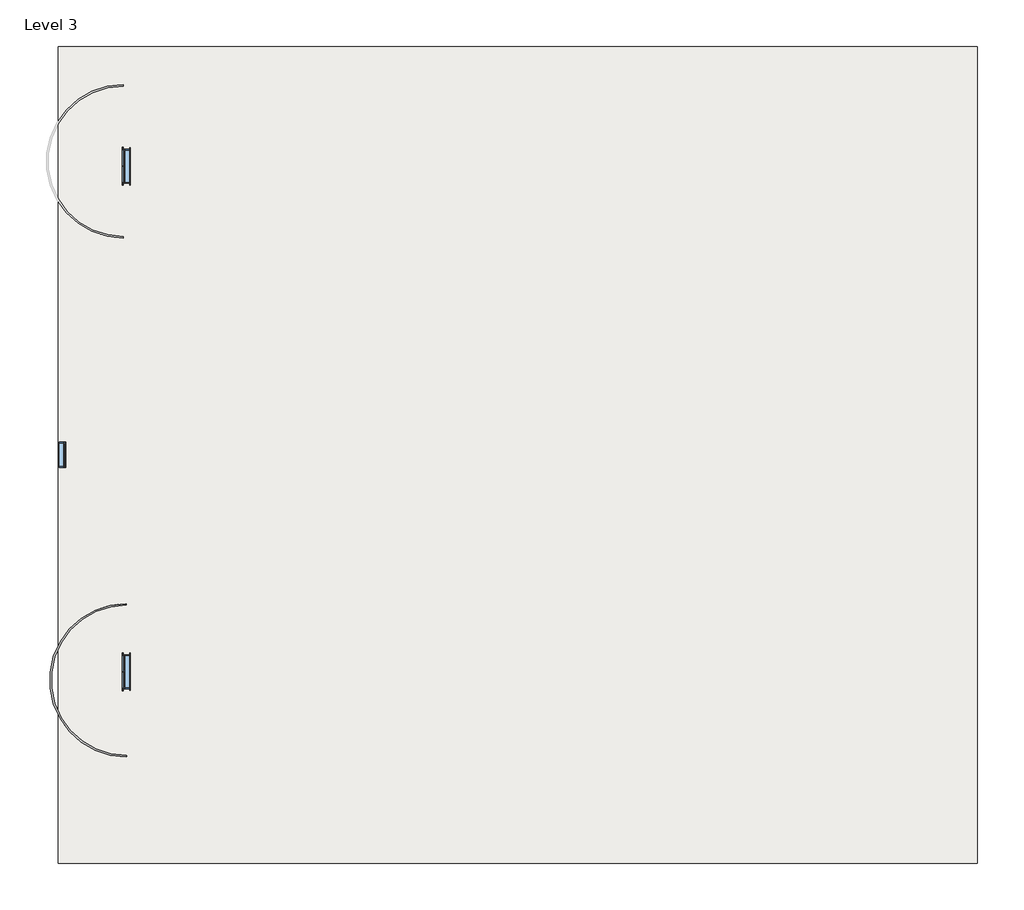
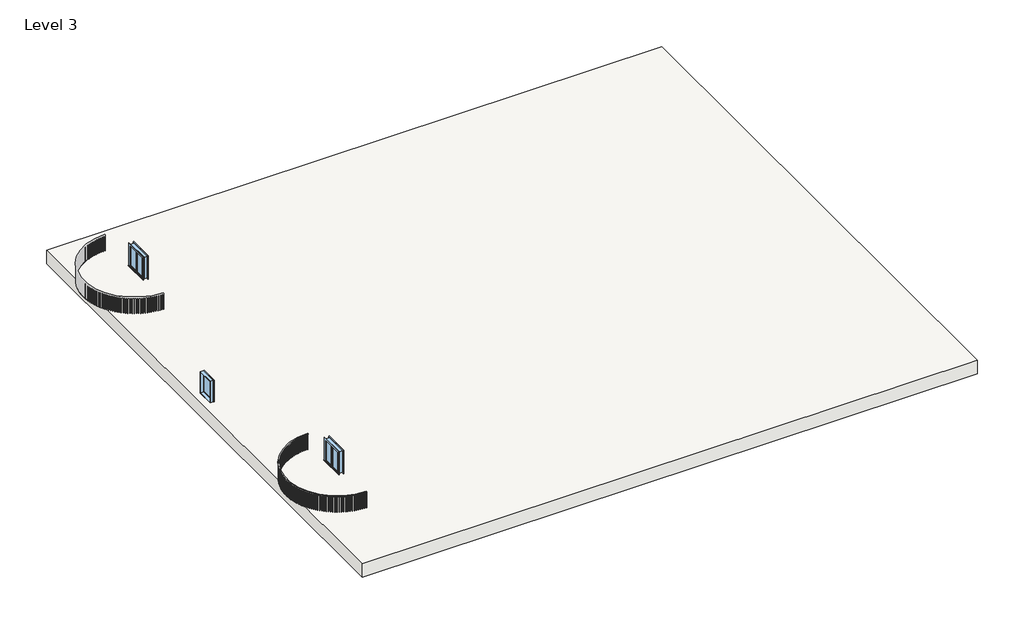
# One storey, part 1 of 2: 3 windows, 1 railing, 1 slab.
"""IFC4 building model written with IfcOpenShell, lengths in millimetres."""

from ifc_helpers import new_model, si_unit, point, frame, frame_2d, origin, place, context, project, spatial, polyline, circle_curve, trimmed, segment, composite_curve, outline, extrude, transform, mapped, element, save
from components import window_534dcd48, window_c1f32544

model = new_model("IFC4")

# Units and contexts
model_context = context("Model", 3, world=origin())
ifc_project = project(units=[si_unit("LENGTHUNIT", "METRE", prefix="MILLI")], contexts=[model_context])

# Site, building, storey
site = spatial("IfcSite", under=ifc_project)
building = spatial("IfcBuilding", under=site)
storey = spatial("IfcBuildingStorey", under=building, Name="Level 3", Elevation=6096.0)

# Railing
placement = place(None, origin())
element("IfcRailing", 1, ObjectType="Handrail - Rectangular", at=placement, inside=storey, context=model_context, shape_type="SweptSolid", body=[
    extrude(outline(composite_curve([segment(trimmed(circle_curve(frame_2d((-15613.8723021, -8267.0443987)), 2743.2), [point((-15613.8723021, -11010.2443987))], [point((-15613.8723021, -5523.8443987))], False, "CARTESIAN"), True, "CONTINUOUS"), segment(polyline([(-15613.8723021, -5523.8443987), (-15613.8723021, -5574.6443987)]), True, "CONTINUOUS"), segment(trimmed(circle_curve(frame_2d((-15613.8723021, -8267.0443987)), 2692.4), [point((-15613.8723021, -5574.6443987))], [point((-15613.8723021, -10959.4443987))], True, "CARTESIAN"), True, "CONTINUOUS"), segment(polyline([(-15613.8723021, -10959.4443987), (-15613.8723021, -11010.2443987)]), True, "CONTINUOUS")], self_intersect=False)), frame((0.0, 0.0, 6959.6), z_axis=(0.0, 0.0, 1.0), x_axis=(1.0, 0.0, 0.0)), (0.0, 0.0, 1.0), 50.8),
    extrude(outline(polyline([(-15627.231195, -10994.3533143), (-15627.2044157, -10975.3033331), (-15608.1544345, -10975.3301124), (-15608.1812138, -10994.3800936), (-15627.231195, -10994.3533143)])), frame((0.0, 0.0, 6096.0), z_axis=(0.0, 0.0, 1.0), x_axis=(1.0, 0.0, 0.0)), (0.0, 0.0, 1.0), 863.6),
    extrude(outline(polyline([(-15729.1535895, -10991.9485449), (-15728.414846, -10972.9128742), (-15709.3791753, -10973.6516178), (-15710.1179188, -10992.6872885), (-15729.1535895, -10991.9485449)])), frame((0.0, 0.0, 6096.0), z_axis=(0.0, 0.0, 1.0), x_axis=(1.0, 0.0, 0.0)), (0.0, 0.0, 1.0), 863.6),
    extrude(outline(polyline([(-15830.914897, -10985.7361601), (-15829.4652214, -10966.7413992), (-15810.4704606, -10968.1910747), (-15811.9201361, -10987.1858356), (-15830.914897, -10985.7361601)])), frame((0.0, 0.0, 6096.0), z_axis=(0.0, 0.0, 1.0), x_axis=(1.0, 0.0, 0.0)), (0.0, 0.0, 1.0), 863.6),
    extrude(outline(polyline([(-15932.3729223, -10975.7248406), (-15930.2143405, -10956.7975316), (-15911.2870315, -10958.9561134), (-15913.4456133, -10977.8834224), (-15932.3729223, -10975.7248406)])), frame((0.0, 0.0, 6096.0), z_axis=(0.0, 0.0, 1.0), x_axis=(1.0, 0.0, 0.0)), (0.0, 0.0, 1.0), 863.6),
    extrude(outline(polyline([(-16033.3858942, -10961.9285757), (-16030.5214224, -10943.0951665), (-16011.6880132, -10945.9596384), (-16014.5524851, -10964.7930475), (-16033.3858942, -10961.9285757)])), frame((0.0, 0.0, 6096.0), z_axis=(0.0, 0.0, 1.0), x_axis=(1.0, 0.0, 0.0)), (0.0, 0.0, 1.0), 863.6),
    extrude(outline(polyline([(-16133.8126634, -10944.3666434), (-16130.2463041, -10925.6534507), (-16111.5331114, -10929.2198099), (-16115.0994706, -10947.9330026), (-16133.8126634, -10944.3666434)])), frame((0.0, 0.0, 6096.0), z_axis=(0.0, 0.0, 1.0), x_axis=(1.0, 0.0, 0.0)), (0.0, 0.0, 1.0), 863.6),
    extrude(outline(polyline([(-16233.5128994, -10923.0635838), (-16229.2496362, -10904.4967562), (-16210.6828086, -10908.7600194), (-16214.9460718, -10927.326847), (-16233.5128994, -10923.0635838)])), frame((0.0, 0.0, 6096.0), z_axis=(0.0, 0.0, 1.0), x_axis=(1.0, 0.0, 0.0)), (0.0, 0.0, 1.0), 863.6),
    extrude(outline(polyline([(-16332.3472874, -10898.0491643), (-16327.3930774, -10879.654646), (-16308.9985591, -10884.608856), (-16313.9527691, -10903.0033743), (-16332.3472874, -10898.0491643)])), frame((0.0, 0.0, 6096.0), z_axis=(0.0, 0.0, 1.0), x_axis=(1.0, 0.0, 0.0)), (0.0, 0.0, 1.0), 863.6),
    extrude(outline(polyline([(-16430.1777221, -10869.3583388), (-16424.5394881, -10851.1618331), (-16406.3429824, -10856.8000671), (-16411.9812164, -10874.9965728), (-16430.1777221, -10869.3583388)])), frame((0.0, 0.0, 6096.0), z_axis=(0.0, 0.0, 1.0), x_axis=(1.0, 0.0, 0.0)), (0.0, 0.0, 1.0), 863.6),
    extrude(outline(polyline([(-16526.8675012, -10837.0311978), (-16520.5531216, -10819.0581316), (-16502.5800554, -10825.3725111), (-16508.8944349, -10843.3455773), (-16526.8675012, -10837.0311978)])), frame((0.0, 0.0, 6096.0), z_axis=(0.0, 0.0, 1.0), x_axis=(1.0, 0.0, 0.0)), (0.0, 0.0, 1.0), 863.6),
    extrude(outline(polyline([(-16622.2815163, -10801.1129136), (-16615.2998146, -10783.3884011), (-16597.5753021, -10790.3701028), (-16604.5570038, -10808.0946153), (-16622.2815163, -10801.1129136)])), frame((0.0, 0.0, 6096.0), z_axis=(0.0, 0.0, 1.0), x_axis=(1.0, 0.0, 0.0)), (0.0, 0.0, 1.0), 863.6),
    extrude(outline(polyline([(-16716.2864416, -10761.653676), (-16708.6471735, -10744.2024845), (-16691.1959821, -10751.8417526), (-16698.8352501, -10769.292944), (-16716.2864416, -10761.653676)])), frame((0.0, 0.0, 6096.0), z_axis=(0.0, 0.0, 1.0), x_axis=(1.0, 0.0, 0.0)), (0.0, 0.0, 1.0), 863.6),
    extrude(outline(polyline([(-16808.7509204, -10718.708623), (-16800.4647607, -10701.5551378), (-16783.3112754, -10709.8412975), (-16791.5974352, -10726.9947828), (-16808.7509204, -10718.708623)])), frame((0.0, 0.0, 6096.0), z_axis=(0.0, 0.0, 1.0), x_axis=(1.0, 0.0, 0.0)), (0.0, 0.0, 1.0), 863.6),
    extrude(outline(polyline([(-16899.5457485, -10672.3377634), (-16890.6242756, -10655.5059536), (-16873.7924658, -10664.4274266), (-16882.7139387, -10681.2592364), (-16899.5457485, -10672.3377634)])), frame((0.0, 0.0, 6096.0), z_axis=(0.0, 0.0, 1.0), x_axis=(1.0, 0.0, 0.0)), (0.0, 0.0, 1.0), 863.6),
    extrude(outline(polyline([(-16988.5440547, -10622.6058931), (-16978.9997349, -10606.1192785), (-16962.5131203, -10615.6635983), (-16972.0574401, -10632.1502129), (-16988.5440547, -10622.6058931)])), frame((0.0, 0.0, 6096.0), z_axis=(0.0, 0.0, 1.0), x_axis=(1.0, 0.0, 0.0)), (0.0, 0.0, 1.0), 863.6),
    extrude(outline(polyline([(-17075.621478, -10569.5825043), (-17065.4676481, -10553.4641223), (-17049.3492661, -10563.6179523), (-17059.5030961, -10579.7363343), (-17075.621478, -10569.5825043)])), frame((0.0, 0.0, 6096.0), z_axis=(0.0, 0.0, 1.0), x_axis=(1.0, 0.0, 0.0)), (0.0, 0.0, 1.0), 863.6),
    extrude(outline(polyline([(-17160.656342, -10513.3416887), (-17149.9071902, -10497.6140622), (-17134.1795637, -10508.363214), (-17144.9287154, -10524.0908405), (-17160.656342, -10513.3416887)])), frame((0.0, 0.0, 6096.0), z_axis=(0.0, 0.0, 1.0), x_axis=(1.0, 0.0, 0.0)), (0.0, 0.0, 1.0), 863.6),
    extrude(outline(polyline([(-17243.5298239, -10453.9620338), (-17232.2003705, -10438.6471396), (-17216.8854763, -10449.976593), (-17228.2149296, -10465.2914872), (-17243.5298239, -10453.9620338)])), frame((0.0, 0.0, 6096.0), z_axis=(0.0, 0.0, 1.0), x_axis=(1.0, 0.0, 0.0)), (0.0, 0.0, 1.0), 863.6),
    extrude(outline(polyline([(-17324.1261214, -10391.5265132), (-17312.2321975, -10376.6457513), (-17297.3514357, -10388.5396752), (-17309.2453596, -10403.4204371), (-17324.1261214, -10391.5265132)])), frame((0.0, 0.0, 6096.0), z_axis=(0.0, 0.0, 1.0), x_axis=(1.0, 0.0, 0.0)), (0.0, 0.0, 1.0), 863.6),
    extrude(outline(polyline([(-17402.3326143, -10326.1223703), (-17389.8908397, -10311.6965343), (-17375.4650036, -10324.1383088), (-17387.9067782, -10338.5641449), (-17402.3326143, -10326.1223703)])), frame((0.0, 0.0, 6096.0), z_axis=(0.0, 0.0, 1.0), x_axis=(1.0, 0.0, 0.0)), (0.0, 0.0, 1.0), 863.6),
    extrude(outline(polyline([(-17478.0400213, -10257.840997), (-17465.0677814, -10243.8902446), (-17451.117029, -10256.8624845), (-17464.0892689, -10270.8132369), (-17478.0400213, -10257.840997)])), frame((0.0, 0.0, 6096.0), z_axis=(0.0, 0.0, 1.0), x_axis=(1.0, 0.0, 0.0)), (0.0, 0.0, 1.0), 863.6),
    extrude(outline(polyline([(-17551.1425537, -10186.7778056), (-17537.6579752, -10173.3216307), (-17524.2018003, -10186.8062093), (-17537.6863789, -10200.2623841), (-17551.1425537, -10186.7778056)])), frame((0.0, 0.0, 6096.0), z_axis=(0.0, 0.0, 1.0), x_axis=(1.0, 0.0, 0.0)), (0.0, 0.0, 1.0), 863.6),
    extrude(outline(polyline([(-17621.5380624, -10113.0320953), (-17607.5599877, -10100.0893009), (-17594.6171933, -10114.0673756), (-17608.595268, -10127.01017), (-17621.5380624, -10113.0320953)])), frame((0.0, 0.0, 6096.0), z_axis=(0.0, 0.0, 1.0), x_axis=(1.0, 0.0, 0.0)), (0.0, 0.0, 1.0), 863.6),
    extrude(outline(polyline([(-17689.128181, -10036.7069141), (-17674.6761422, -10024.2955856), (-17662.2648137, -10038.7476243), (-17676.7168525, -10051.1589528), (-17689.128181, -10036.7069141)])), frame((0.0, 0.0, 6096.0), z_axis=(0.0, 0.0, 1.0), x_axis=(1.0, 0.0, 0.0)), (0.0, 0.0, 1.0), 863.6),
    extrude(outline(polyline([(-17753.8184631, -9957.908914), (-17738.9126547, -9946.0463942), (-17727.0501349, -9960.9522026), (-17741.9559433, -9972.8147224), (-17753.8184631, -9957.908914)])), frame((0.0, 0.0, 6096.0), z_axis=(0.0, 0.0, 1.0), x_axis=(1.0, 0.0, 0.0)), (0.0, 0.0, 1.0), 863.6),
    extrude(outline(polyline([(-17815.5185146, -9876.7482026), (-17800.179765, -9865.4510675), (-17788.8826299, -9880.789817), (-17804.2213795, -9892.0869522), (-17815.5185146, -9876.7482026)])), frame((0.0, 0.0, 6096.0), z_axis=(0.0, 0.0, 1.0), x_axis=(1.0, 0.0, 0.0)), (0.0, 0.0, 1.0), 863.6),
    extrude(outline(polyline([(-17874.1421194, -9793.338189), (-17858.3918621, -9782.6222244), (-17847.6758976, -9798.3724817), (-17863.4261549, -9809.0884462), (-17874.1421194, -9793.338189)])), frame((0.0, 0.0, 6096.0), z_axis=(0.0, 0.0, 1.0), x_axis=(1.0, 0.0, 0.0)), (0.0, 0.0, 1.0), 863.6),
    extrude(outline(polyline([(-17929.6073606, -9707.7954251), (-17913.467604, -9697.6756051), (-17903.347784, -9713.8153616), (-17919.4875405, -9723.9351817), (-17929.6073606, -9707.7954251)])), frame((0.0, 0.0, 6096.0), z_axis=(0.0, 0.0, 1.0), x_axis=(1.0, 0.0, 0.0)), (0.0, 0.0, 1.0), 863.6),
    extrude(outline(polyline([(-17981.8367343, -9620.2394434), (-17965.3300312, -9610.7299086), (-17955.8204964, -9627.2366117), (-17972.3271995, -9636.7461465), (-17981.8367343, -9620.2394434)])), frame((0.0, 0.0, 6096.0), z_axis=(0.0, 0.0, 1.0), x_axis=(1.0, 0.0, 0.0)), (0.0, 0.0, 1.0), 863.6),
    extrude(outline(polyline([(-18030.7572585, -9530.7925891), (-18013.9066743, -9521.9066277), (-18005.0207128, -9538.7572119), (-18021.871297, -9547.6431733), (-18030.7572585, -9530.7925891)])), frame((0.0, 0.0, 6096.0), z_axis=(0.0, 0.0, 1.0), x_axis=(1.0, 0.0, 0.0)), (0.0, 0.0, 1.0), 863.6),
    extrude(outline(polyline([(-18076.3005745, -9439.5798499), (-18059.1296552, -9431.3298785), (-18050.8796837, -9448.5007978), (-18068.0506031, -9456.7507693), (-18076.3005745, -9439.5798499)])), frame((0.0, 0.0, 6096.0), z_axis=(0.0, 0.0, 1.0), x_axis=(1.0, 0.0, 0.0)), (0.0, 0.0, 1.0), 863.6),
    extrude(outline(polyline([(-18118.4030429, -9346.728681), (-18100.9357821, -9339.1262276), (-18093.3333287, -9356.5934885), (-18110.8005895, -9364.1959419), (-18118.4030429, -9346.728681)])), frame((0.0, 0.0, 6096.0), z_axis=(0.0, 0.0, 1.0), x_axis=(1.0, 0.0, 0.0)), (0.0, 0.0, 1.0), 863.6),
    extrude(outline(polyline([(-18157.0058323, -9252.3688268), (-18139.2666376, -9245.4245147), (-18132.3223254, -9263.1637094), (-18150.0615201, -9270.1080215), (-18157.0058323, -9252.3688268)])), frame((0.0, 0.0, 6096.0), z_axis=(0.0, 0.0, 1.0), x_axis=(1.0, 0.0, 0.0)), (0.0, 0.0, 1.0), 863.6),
    extrude(outline(polyline([(-18192.0550015, -9156.6321402), (-18174.0686606, -9150.3556729), (-18167.7921932, -9168.3420137), (-18185.7785341, -9174.6184811), (-18192.0550015, -9156.6321402)])), frame((0.0, 0.0, 6096.0), z_axis=(0.0, 0.0, 1.0), x_axis=(1.0, 0.0, 0.0)), (0.0, 0.0, 1.0), 863.6),
    extrude(outline(polyline([(-18223.5015748, -9059.6523978), (-18205.2932208, -9054.0525456), (-18199.6933686, -9072.2608996), (-18217.9017226, -9077.8607518), (-18223.5015748, -9059.6523978)])), frame((0.0, 0.0, 6096.0), z_axis=(0.0, 0.0, 1.0), x_axis=(1.0, 0.0, 0.0)), (0.0, 0.0, 1.0), 863.6),
    extrude(outline(polyline([(-18251.3016108, -8961.5651131), (-18232.8966869, -8956.6497009), (-18227.9812748, -8975.0546248), (-18246.3861986, -8979.970037), (-18251.3016108, -8961.5651131)])), frame((0.0, 0.0, 6096.0), z_axis=(0.0, 0.0, 1.0), x_axis=(1.0, 0.0, 0.0)), (0.0, 0.0, 1.0), 863.6),
    extrude(outline(polyline([(-18275.4162634, -8862.5073473), (-18256.8404876, -8858.2832437), (-18252.6163839, -8876.8590196), (-18271.1921598, -8881.0831232), (-18275.4162634, -8862.5073473)])), frame((0.0, 0.0, 6096.0), z_axis=(0.0, 0.0, 1.0), x_axis=(1.0, 0.0, 0.0)), (0.0, 0.0, 1.0), 863.6),
    extrude(outline(polyline([(-18295.8118362, -8762.6175179), (-18277.0911651, -8759.0906253), (-18273.5642725, -8777.8112965), (-18292.2849436, -8781.338189), (-18295.8118362, -8762.6175179)])), frame((0.0, 0.0, 6096.0), z_axis=(0.0, 0.0, 1.0), x_axis=(1.0, 0.0, 0.0)), (0.0, 0.0, 1.0), 863.6),
    extrude(outline(polyline([(-18312.4598298, -8662.0352047), (-18293.6204224, -8659.2104514), (-18290.7956691, -8678.0498587), (-18309.6350765, -8680.874612), (-18312.4598298, -8662.0352047)])), frame((0.0, 0.0, 6096.0), z_axis=(0.0, 0.0, 1.0), x_axis=(1.0, 0.0, 0.0)), (0.0, 0.0, 1.0), 863.6),
    extrude(outline(polyline([(-18325.3369811, -8560.9009553), (-18306.4051626, -8558.7822885), (-18304.2864958, -8577.714107), (-18323.2183143, -8579.8327738), (-18325.3369811, -8560.9009553)])), frame((0.0, 0.0, 6096.0), z_axis=(0.0, 0.0, 1.0), x_axis=(1.0, 0.0, 0.0)), (0.0, 0.0, 1.0), 863.6),
    extrude(outline(polyline([(-18334.4252965, -8459.3560886), (-18315.427521, -8457.9464688), (-18314.0179011, -8476.9442442), (-18333.0156766, -8478.3538641), (-18334.4252965, -8459.3560886)])), frame((0.0, 0.0, 6096.0), z_axis=(0.0, 0.0, 1.0), x_axis=(1.0, 0.0, 0.0)), (0.0, 0.0, 1.0), 863.6),
    extrude(outline(polyline([(-18339.7120764, -8357.5424973), (-18320.6748904, -8356.8438941), (-18319.9762872, -8375.8810802), (-18339.0134732, -8376.5796834), (-18339.7120764, -8357.5424973)])), frame((0.0, 0.0, 6096.0), z_axis=(0.0, 0.0, 1.0), x_axis=(1.0, 0.0, 0.0)), (0.0, 0.0, 1.0), 863.6),
    extrude(outline(polyline([(-18341.1899336, -8255.6024494), (-18322.1399383, -8255.6158391), (-18322.1533279, -8274.6658344), (-18341.2033232, -8274.6524447), (-18341.1899336, -8255.6024494)])), frame((0.0, 0.0, 6096.0), z_axis=(0.0, 0.0, 1.0), x_axis=(1.0, 0.0, 0.0)), (0.0, 0.0, 1.0), 863.6),
    extrude(outline(polyline([(-18338.8568028, -8153.6783898), (-18319.8206176, -8154.4037536), (-18320.5459814, -8173.4399388), (-18339.5821666, -8172.7145751), (-18338.8568028, -8153.6783898)])), frame((0.0, 0.0, 6096.0), z_axis=(0.0, 0.0, 1.0), x_axis=(1.0, 0.0, 0.0)), (0.0, 0.0, 1.0), 863.6),
    extrude(outline(polyline([(-18332.7159444, -8051.912741), (-18313.7201692, -8053.3490654), (-18315.1564936, -8072.3448405), (-18334.1522687, -8070.9085161), (-18332.7159444, -8051.912741)])), frame((0.0, 0.0, 6096.0), z_axis=(0.0, 0.0, 1.0), x_axis=(1.0, 0.0, 0.0)), (0.0, 0.0, 1.0), 863.6),
    extrude(outline(polyline([(-18322.775939, -7950.4477041), (-18303.8471175, -7952.592982), (-18305.9923954, -7971.5218035), (-18324.9212169, -7969.3765256), (-18322.775939, -7950.4477041)])), frame((0.0, 0.0, 6096.0), z_axis=(0.0, 0.0, 1.0), x_axis=(1.0, 0.0, 0.0)), (0.0, 0.0, 1.0), 863.6),
    extrude(outline(polyline([(-18309.0506764, -7849.4250602), (-18290.2152585, -7852.2762939), (-18293.0664923, -7871.1117118), (-18311.9019101, -7868.260478), (-18309.0506764, -7849.4250602)])), frame((0.0, 0.0, 6096.0), z_axis=(0.0, 0.0, 1.0), x_axis=(1.0, 0.0, 0.0)), (0.0, 0.0, 1.0), 863.6),
    extrude(outline(polyline([(-18291.5593353, -7748.9859721), (-18272.8436405, -7752.5391776), (-18276.396846, -7771.2548723), (-18295.1125408, -7767.7016669), (-18291.5593353, -7748.9859721)])), frame((0.0, 0.0, 6096.0), z_axis=(0.0, 0.0, 1.0), x_axis=(1.0, 0.0, 0.0)), (0.0, 0.0, 1.0), 863.6),
    extrude(outline(polyline([(-18270.3263571, -7649.2707874), (-18251.7565376, -7653.5209995), (-18256.0067497, -7672.0908191), (-18274.5765692, -7667.8406069), (-18270.3263571, -7649.2707874)])), frame((0.0, 0.0, 6096.0), z_axis=(0.0, 0.0, 1.0), x_axis=(1.0, 0.0, 0.0)), (0.0, 0.0, 1.0), 863.6),
    extrude(outline(polyline([(-18245.3814115, -7550.418842), (-18226.9834156, -7555.3601218), (-18231.9246954, -7573.7581178), (-18250.3226913, -7568.816838), (-18245.3814115, -7550.418842)])), frame((0.0, 0.0, 6096.0), z_axis=(0.0, 0.0, 1.0), x_axis=(1.0, 0.0, 0.0)), (0.0, 0.0, 1.0), 863.6),
    extrude(outline(polyline([(-18216.7593549, -7452.5682656), (-18198.5588909, -7458.1937085), (-18204.1843337, -7476.3941726), (-18222.3847978, -7470.7687297), (-18216.7593549, -7452.5682656)])), frame((0.0, 0.0, 6096.0), z_axis=(0.0, 0.0, 1.0), x_axis=(1.0, 0.0, 0.0)), (0.0, 0.0, 1.0), 863.6),
    extrude(outline(polyline([(-18184.5001822, -7355.8557887), (-18166.5226822, -7362.1575339), (-18172.8244275, -7380.1350339), (-18190.8019275, -7373.8332887), (-18184.5001822, -7355.8557887)])), frame((0.0, 0.0, 6096.0), z_axis=(0.0, 0.0, 1.0), x_axis=(1.0, 0.0, 0.0)), (0.0, 0.0, 1.0), 863.6),
    extrude(outline(polyline([(-18148.6489704, -7260.4165513), (-18130.9195551, -7267.3857933), (-18137.888797, -7285.1152086), (-18155.6182123, -7278.1459666), (-18148.6489704, -7260.4165513)])), frame((0.0, 0.0, 6096.0), z_axis=(0.0, 0.0, 1.0), x_axis=(1.0, 0.0, 0.0)), (0.0, 0.0, 1.0), 863.6),
    extrude(outline(polyline([(-18109.2558157, -7166.3839145), (-18091.7992591, -7174.0109148), (-18099.4262594, -7191.4674713), (-18116.8828159, -7183.8404711), (-18109.2558157, -7166.3839145)])), frame((0.0, 0.0, 6096.0), z_axis=(0.0, 0.0, 1.0), x_axis=(1.0, 0.0, 0.0)), (0.0, 0.0, 1.0), 863.6),
    extrude(outline(polyline([(-18066.3757637, -7073.8892738), (-18049.2164586, -7082.1633749), (-18057.4905597, -7099.32268), (-18074.6498648, -7091.0485789), (-18066.3757637, -7073.8892738)])), frame((0.0, 0.0, 6096.0), z_axis=(0.0, 0.0, 1.0), x_axis=(1.0, 0.0, 0.0)), (0.0, 0.0, 1.0), 863.6),
    extrude(outline(polyline([(-18020.0687324, -6983.0618755), (-18003.2306562, -6991.9715157), (-18012.1402963, -7008.8095919), (-18028.9783726, -6999.8999518), (-18020.0687324, -6983.0618755)])), frame((0.0, 0.0, 6096.0), z_axis=(0.0, 0.0, 1.0), x_axis=(1.0, 0.0, 0.0)), (0.0, 0.0, 1.0), 863.6),
    extrude(outline(polyline([(-17970.3994285, -6894.0286364), (-17953.9061096, -6903.5613658), (-17963.4388391, -6920.0546848), (-17979.932158, -6910.5219553), (-17970.3994285, -6894.0286364)])), frame((0.0, 0.0, 6096.0), z_axis=(0.0, 0.0, 1.0), x_axis=(1.0, 0.0, 0.0)), (0.0, 0.0, 1.0), 863.6),
    extrude(outline(polyline([(-17917.4372568, -6806.913966), (-17901.311742, -6817.0564643), (-17911.4542403, -6833.1819791), (-17927.5797552, -6823.0394808), (-17917.4372568, -6806.913966)])), frame((0.0, 0.0, 6096.0), z_axis=(0.0, 0.0, 1.0), x_axis=(1.0, 0.0, 0.0)), (0.0, 0.0, 1.0), 863.6),
    extrude(outline(polyline([(-17861.2562235, -6721.8395932), (-17845.5210456, -6732.5776878), (-17856.2591402, -6748.3128657), (-17871.9943181, -6737.5747711), (-17861.2562235, -6721.8395932)])), frame((0.0, 0.0, 6096.0), z_axis=(0.0, 0.0, 1.0), x_axis=(1.0, 0.0, 0.0)), (0.0, 0.0, 1.0), 863.6),
    extrude(outline(polyline([(-17801.9348324, -6638.9243956), (-17786.6119788, -6650.2430818), (-17797.9306651, -6665.5659354), (-17813.2535187, -6654.2472492), (-17801.9348324, -6638.9243956)])), frame((0.0, 0.0, 6096.0), z_axis=(0.0, 0.0, 1.0), x_axis=(1.0, 0.0, 0.0)), (0.0, 0.0, 1.0), 863.6),
    extrude(outline(polyline([(-17739.5559758, -6558.284234), (-17724.6668577, -6570.1676957), (-17736.5503195, -6585.0568138), (-17751.4394375, -6573.1733521), (-17739.5559758, -6558.284234)])), frame((0.0, 0.0, 6096.0), z_axis=(0.0, 0.0, 1.0), x_axis=(1.0, 0.0, 0.0)), (0.0, 0.0, 1.0), 863.6),
    extrude(outline(polyline([(-17674.206818, -6480.03179), (-17659.7722406, -6492.463422), (-17672.2038726, -6506.8979994), (-17686.63845, -6494.4663674), (-17674.206818, -6480.03179)])), frame((0.0, 0.0, 6096.0), z_axis=(0.0, 0.0, 1.0), x_axis=(1.0, 0.0, 0.0)), (0.0, 0.0, 1.0), 863.6),
    extrude(outline(polyline([(-17605.978674, -6404.2764087), (-17592.0188072, -6417.2388399), (-17604.9812384, -6431.1987066), (-17618.9411051, -6418.2362755), (-17605.978674, -6404.2764087)])), frame((0.0, 0.0, 6096.0), z_axis=(0.0, 0.0, 1.0), x_axis=(1.0, 0.0, 0.0)), (0.0, 0.0, 1.0), 863.6),
    extrude(outline(polyline([(-17534.9668816, -6331.1239463), (-17521.5012322, -6344.5990636), (-17534.9763495, -6358.064713), (-17548.4419989, -6344.5895957), (-17534.9668816, -6331.1239463)])), frame((0.0, 0.0, 6096.0), z_axis=(0.0, 0.0, 1.0), x_axis=(1.0, 0.0, 0.0)), (0.0, 0.0, 1.0), 863.6),
    extrude(outline(polyline([(-17461.2706683, -6260.6766214), (-17448.3180524, -6274.6455956), (-17462.2870265, -6287.5982116), (-17475.2396425, -6273.6292374), (-17461.2706683, -6260.6766214)])), frame((0.0, 0.0, 6096.0), z_axis=(0.0, 0.0, 1.0), x_axis=(1.0, 0.0, 0.0)), (0.0, 0.0, 1.0), 863.6),
    extrude(outline(polyline([(-17384.9930129, -6193.032873), (-17372.5715296, -6207.4761846), (-17387.0148412, -6219.897668), (-17399.4363246, -6205.4543563), (-17384.9930129, -6193.032873)])), frame((0.0, 0.0, 6096.0), z_axis=(0.0, 0.0, 1.0), x_axis=(1.0, 0.0, 0.0)), (0.0, 0.0, 1.0), 863.6),
    extrude(outline(polyline([(-17306.2405011, -6128.2872222), (-17294.3675074, -6143.1846891), (-17309.2649743, -6155.0576828), (-17321.137968, -6140.1602159), (-17306.2405011, -6128.2872222)])), frame((0.0, 0.0, 6096.0), z_axis=(0.0, 0.0, 1.0), x_axis=(1.0, 0.0, 0.0)), (0.0, 0.0, 1.0), 863.6),
    extrude(outline(polyline([(-17225.1231768, -6066.5301406), (-17213.8152633, -6081.860946), (-17229.1460687, -6093.1688594), (-17240.4539822, -6077.8380541), (-17225.1231768, -6066.5301406)])), frame((0.0, 0.0, 6096.0), z_axis=(0.0, 0.0, 1.0), x_axis=(1.0, 0.0, 0.0)), (0.0, 0.0, 1.0), 863.6),
    extrude(outline(polyline([(-17141.7543884, -6007.847924), (-17131.0273562, -6023.5906455), (-17146.7700777, -6034.3176777), (-17157.4971099, -6018.5749562), (-17141.7543884, -6007.847924)])), frame((0.0, 0.0, 6096.0), z_axis=(0.0, 0.0, 1.0), x_axis=(1.0, 0.0, 0.0)), (0.0, 0.0, 1.0), 863.6),
    extrude(outline(polyline([(-17056.2506305, -5952.3225712), (-17046.1194688, -5968.4552108), (-17062.2521085, -5978.5863725), (-17072.3832702, -5962.4537328), (-17056.2506305, -5952.3225712)])), frame((0.0, 0.0, 6096.0), z_axis=(0.0, 0.0, 1.0), x_axis=(1.0, 0.0, 0.0)), (0.0, 0.0, 1.0), 863.6),
    extrude(outline(polyline([(-16968.7313808, -5900.03167), (-16959.2102463, -5916.5316851), (-16975.7102614, -5926.0528195), (-16985.2313959, -5909.5528044), (-16968.7313808, -5900.03167)])), frame((0.0, 0.0, 6096.0), z_axis=(0.0, 0.0, 1.0), x_axis=(1.0, 0.0, 0.0)), (0.0, 0.0, 1.0), 863.6),
    extrude(outline(polyline([(-16879.3189333, -5851.0482885), (-16870.4211303, -5867.8926229), (-16887.2654647, -5876.7904259), (-16896.1632677, -5859.9460915), (-16879.3189333, -5851.0482885)])), frame((0.0, 0.0, 6096.0), z_axis=(0.0, 0.0, 1.0), x_axis=(1.0, 0.0, 0.0)), (0.0, 0.0, 1.0), 863.6),
    extrude(outline(polyline([(-16788.1382277, -5805.4408731), (-16779.8761894, -5822.6059896), (-16797.0413058, -5830.8680279), (-16805.3033441, -5813.7029114), (-16788.1382277, -5805.4408731)])), frame((0.0, 0.0, 6096.0), z_axis=(0.0, 0.0, 1.0), x_axis=(1.0, 0.0, 0.0)), (0.0, 0.0, 1.0), 863.6),
    extrude(outline(polyline([(-16695.3166742, -5763.2731529), (-16687.7019455, -5780.7350659), (-16705.1638585, -5788.3497946), (-16712.7785872, -5770.8878816), (-16695.3166742, -5763.2731529)])), frame((0.0, 0.0, 6096.0), z_axis=(0.0, 0.0, 1.0), x_axis=(1.0, 0.0, 0.0)), (0.0, 0.0, 1.0), 863.6),
    extrude(outline(polyline([(-16600.983976, -5724.6040505), (-16594.0271973, -5742.3383598), (-16611.7615066, -5749.2951386), (-16618.7182854, -5731.5608292), (-16600.983976, -5724.6040505)])), frame((0.0, 0.0, 6096.0), z_axis=(0.0, 0.0, 1.0), x_axis=(1.0, 0.0, 0.0)), (0.0, 0.0, 1.0), 863.6),
    extrude(outline(polyline([(-16505.271948, -5689.4875996), (-16498.9828402, -5707.4695245), (-16516.9647651, -5713.7586324), (-16523.2538729, -5695.7767075), (-16505.271948, -5689.4875996)])), frame((0.0, 0.0, 6096.0), z_axis=(0.0, 0.0, 1.0), x_axis=(1.0, 0.0, 0.0)), (0.0, 0.0, 1.0), 863.6),
    extrude(outline(polyline([(-16408.3143324, -5657.97287), (-16402.7016834, -5676.1772836), (-16420.906097, -5681.7899325), (-16426.5187459, -5663.5855189), (-16408.3143324, -5657.97287)])), frame((0.0, 0.0, 6096.0), z_axis=(0.0, 0.0, 1.0), x_axis=(1.0, 0.0, 0.0)), (0.0, 0.0, 1.0), 863.6),
    extrude(outline(polyline([(-16310.2466117, -5630.1038984), (-16305.3182645, -5648.5053628), (-16323.7197289, -5653.43371), (-16328.6480761, -5635.0322456), (-16310.2466117, -5630.1038984)])), frame((0.0, 0.0, 6096.0), z_axis=(0.0, 0.0, 1.0), x_axis=(1.0, 0.0, 0.0)), (0.0, 0.0, 1.0), 863.6),
    extrude(outline(polyline([(-16211.2058198, -5605.9196271), (-16206.9686609, -5624.4924294), (-16225.5414632, -5628.7295883), (-16229.7786221, -5610.1567861), (-16211.2058198, -5605.9196271)])), frame((0.0, 0.0, 6096.0), z_axis=(0.0, 0.0, 1.0), x_axis=(1.0, 0.0, 0.0)), (0.0, 0.0, 1.0), 863.6),
    extrude(outline(polyline([(-16111.3303505, -5585.4538499), (-16107.7903006, -5604.1720375), (-16126.5084882, -5607.7120874), (-16130.048538, -5588.9938998), (-16111.3303505, -5585.4538499)])), frame((0.0, 0.0, 6096.0), z_axis=(0.0, 0.0, 1.0), x_axis=(1.0, 0.0, 0.0)), (0.0, 0.0, 1.0), 863.6),
    extrude(outline(polyline([(-16010.7597634, -5568.7351643), (-16007.9217692, -5587.5725816), (-16026.7591865, -5590.4105758), (-16029.5971807, -5571.5731585), (-16010.7597634, -5568.7351643)])), frame((0.0, 0.0, 6096.0), z_axis=(0.0, 0.0, 1.0), x_axis=(1.0, 0.0, 0.0)), (0.0, 0.0, 1.0), 863.6),
    extrude(outline(polyline([(-15909.63459, -5555.7869321), (-15907.5026171, -5574.7172567), (-15926.4329418, -5576.8492296), (-15928.5649146, -5557.918905), (-15909.63459, -5555.7869321)])), frame((0.0, 0.0, 6096.0), z_axis=(0.0, 0.0, 1.0), x_axis=(1.0, 0.0, 0.0)), (0.0, 0.0, 1.0), 863.6),
    extrude(outline(polyline([(-15808.0961363, -5546.6272462), (-15806.6731638, -5565.6240262), (-15825.6699438, -5567.0469987), (-15827.0929163, -5548.0502187), (-15808.0961363, -5546.6272462)])), frame((0.0, 0.0, 6096.0), z_axis=(0.0, 0.0, 1.0), x_axis=(1.0, 0.0, 0.0)), (0.0, 0.0, 1.0), 863.6),
    extrude(outline(polyline([(-15706.286286, -5541.268906), (-15705.5743024, -5560.3055963), (-15724.6109927, -5561.01758), (-15725.3229764, -5541.9808896), (-15706.286286, -5541.268906)])), frame((0.0, 0.0, 6096.0), z_axis=(0.0, 0.0, 1.0), x_axis=(1.0, 0.0, 0.0)), (0.0, 0.0, 1.0), 863.6),
    extrude(outline(polyline([(-15632.955606, -10994.3192673), (-15632.8888422, -10975.2693843), (-15613.8389591, -10975.3361482), (-15613.905723, -10994.3860312), (-15632.955606, -10994.3192673)])), frame((0.0, 0.0, 6096.0), z_axis=(0.0, 0.0, 1.0), x_axis=(1.0, 0.0, 0.0)), (0.0, 0.0, 1.0), 863.6),
    extrude(outline(polyline([(-15613.905723, -5539.7027662), (-15613.8389591, -5558.7526493), (-15632.8888422, -5558.8194131), (-15632.955606, -5539.7695301), (-15613.905723, -5539.7027662)])), frame((0.0, 0.0, 6096.0), z_axis=(0.0, 0.0, 1.0), x_axis=(1.0, 0.0, 0.0)), (0.0, 0.0, 1.0), 863.6),
])

# Slab
element("IfcSlab", 2, ObjectType="Generic - 12\"", at=placement, inside=storey, context=model_context, shape_type="SweptSolid", body=[
    extrude(outline(polyline([(14866.1276979, 14440.5556013), (14866.1276979, -14820.2443987), (-18052.2723021, -14820.2443987), (-18052.2723021, 14440.5556013), (14866.1276979, 14440.5556013)])), frame((0.0, 0.0, 5334.0), z_axis=(0.0, 0.0, 1.0), x_axis=(1.0, 0.0, 0.0)), (0.0, 0.0, 1.0), 762.0),
])

# Windows
window_shape = window_534dcd48(model_context)
element("IfcWindow", 3, ObjectType="Casement Dbl with Trim : 48\" x 48\"", at=placement, inside=storey, context=model_context, shape_type="MappedRepresentation", body=[
    mapped(window_shape, transform((-15594.8223021, 10147.9556013, 5701.7919963), x_axis=(0.0, 1.0, 0.0), y_axis=(-1.0, 0.0, 0.0), z_axis=(0.0, 0.0, 1.0))),
])
element("IfcWindow", 4, ObjectType="Casement Dbl with Trim : 48\" x 48\"", at=placement, inside=storey, context=model_context, shape_type="MappedRepresentation", body=[
    mapped(window_shape, transform((-15594.8223021, -7962.2443987, 5679.7755614), x_axis=(0.0, 1.0, 0.0), y_axis=(-1.0, 0.0, 0.0), z_axis=(0.0, 0.0, 1.0))),
])
window_2_shape = window_c1f32544(model_context)
element("IfcWindow", 5, ObjectType="Fixed : 36\" x 48\"", at=placement, inside=storey, context=model_context, shape_type="MappedRepresentation", body=[
    mapped(window_2_shape, transform((-17899.8723021, -227.9443987, 5678.3274554), x_axis=(0.0, -1.0, 0.0), y_axis=(1.0, 0.0, 0.0), z_axis=(0.0, 0.0, 1.0))),
])

save(model, "model.ifc")

# Revit data of these elements
# Type "Handrail - Rectangular"
#   Assembly Code = "C2010400"
#   built-in parameter 1008612 = 0.0416667 (stored number, unit not read)
#   built-in parameter 1008611 = 0.0416667 (stored number, unit not read)
#   built-in parameter 1008609 = 0.333333 (stored number, unit not read)
#   built-in parameter 1008604 = 0.166667 (stored number, unit not read)
#   built-in parameter 1008603 = 0.166667 (stored number, unit not read)
#   Railing Height = 3' - 0"
#   built-in parameter 1008630 = 2
#   built-in parameter 1008610 = 2
#   built-in parameter 1008618 = Baluster - Square : 3/4"
# Type "Generic - 12\""
#   Assembly Code = "B1010"
#   Function = 0
#   Layers, outside or top first: 2' - 6" no material (function 1)
# Type "Casement Dbl with Trim : 48\" x 48\""
#   Type Mark = "19"
#   Construction Type Id = "GSP4R"
#   Assembly Code = "B2020100"
#   Analytic Construction = "1/8 in Pilkington single glazing"
#   Visual Light Transmittance = 0.9
#   Solar Heat Gain Coefficient = 0.78
#   Heat Transfer Coefficient (U) = 0.6496 BTU/(h·ft²·°F)
#   Height = 4' - 0"
#   Default Sill Height = 3' - 0"
#   Trim Projection - Ext. = 0' - 0 1/2"
#   Trim Projection - Int. = 0' - 0 3/4"
#   Trim Width - Exterior = 0' - 3 1/2"
#   Trim Width - Interior = 0' - 3 1/2"
#   Width = 4' - 0"
#   Window Inset = 0' - 0 3/4"
#   Define Thermal Properties by = 1
#   Glass Pane Material = Glass
#   Sash Material = Sash
#   Trim Exterior Material = Trim
#   Trim Interior Material = Trim
#   Wall Closure = (empty or 0)
# Type "Fixed : 36\" x 48\""
#   Type Mark = "1"
#   Construction Type Id = "GSP4R"
#   Assembly Code = "B2020100"
#   Analytic Construction = "1/8 in Pilkington single glazing"
#   Visual Light Transmittance = 0.9
#   Solar Heat Gain Coefficient = 0.78
#   Heat Transfer Coefficient (U) = 0.6496 BTU/(h·ft²·°F)
#   Height = 4' - 0"
#   Default Sill Height = 3' - 0"
#   Width = 3' - 0"
#   Window Inset = 0' - 0 3/4"
#   Define Thermal Properties by = 1
#   Glass Pane Material = Glass
#   Sash Material = Sash
#   Wall Closure = (empty or 0)
# Element 1 (IfcRailing, "Handrail - Rectangular")
#   Phase Created = New Construction
# Element 2 (IfcSlab, "Generic - 12\"")
#   Height Offset From Level = 0' - 0"
#   Phase Created = New Construction
#   Materials on its faces: "Default Floor"
# Element 3 (IfcWindow, "Casement Dbl with Trim : 48\" x 48\"")
#   Mark = "7"
#   Phase Created = New Construction
#   Materials on its faces: "Sash", "Trim", "Glass"
# Element 4 (IfcWindow, "Casement Dbl with Trim : 48\" x 48\"")
#   Mark = "10"
#   Phase Created = New Construction
#   Materials on its faces: "Sash", "Trim", "Glass"
# Element 5 (IfcWindow, "Fixed : 36\" x 48\"")
#   Mark = "22"
#   Phase Created = New Construction
#   Materials on its faces: "Sash", "Glass"
# Materials
#   "Glass": class "Glass", colour RGB 0 128 192, transparency 0.75, Description = "Soda Lime Glass", Cost = 0
#   "Sash": class "Wood", colour RGB 224 178 126, transparency 0
#   "Trim": class "Wood", colour RGB 224 178 126, transparency 0
#   "Default Floor": colour RGB 128 128 128, transparency 0
